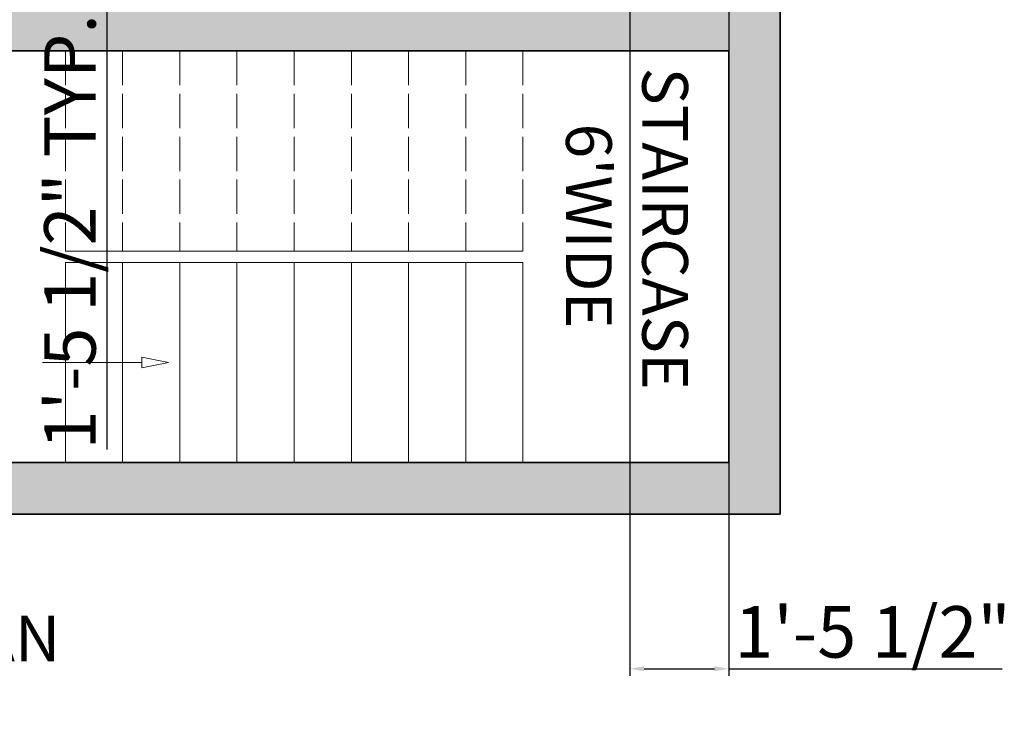
# Model space of a CAD drawing. Units: inches. Extents: x 3592 to 4861, y 1650 to 2243.
# Tile 11 of 30: x 4265 to 4438, y 1650 to 1772. Entities that reach past the tile are written whole.
import ezdxf

# ---------------------------------------------------------------- set-up
doc = ezdxf.new("R2010")
doc.units = ezdxf.units.IN
doc.linetypes.add('ACAD_ISO02W100', pattern=[15, 12, -3])
for name, color, linetype, lineweight in [('A-ANNO-DIMS', 2, 'Continuous', 13), ('A-ANNO-SYMB', 7, 'Continuous', 18), ('A-ANNO-TEXT', 7, 'Continuous', 25), ('A-AREA-IDEN', 7, 'Continuous', 18), ('A-FLOR-STRS', 7, 'Continuous', 18), ('A-FLOR-STRS-OVHD', 8, 'ACAD_ISO02W100', 13), ('A-WALL', 7, 'Continuous', 35)]:
    doc.layers.add(name, color=color, linetype=linetype, lineweight=lineweight)
doc.layers.add('A-WALL-PATT', color=252, linetype='Continuous', lineweight=13, true_color=0x939598)
doc.styles.get("Standard").update_dxf_attribs({"font": 'arial.ttf'})
doc.dimstyles.new('ISO-25', dxfattribs={"dimtxt": 9, "dimasz": 2.5, "dimexe": 1.25, "dimexo": 0.625, "dimtad": 1, "dimlunit": 3, "dimtxsty": 'Standard', "dimcen": 2.5, "dimadec": 0, "dimazin": 0, "dimtfac": 1, "dimtmove": 0, "dimatfit": 3, "dimfxl": 1, "dimarcsym": 0})

# ---------------------------------------------------------------- blocks, each defined once
blk = doc.blocks.new('ARROW-STAIR-DIRECTION')
blk.add_line((0, 0.94), (17.38, 0.94))
blk.add_lwpolyline([(22.04, 0.94), (17.38, 1.89), (17.38, 0)], close=True)
blk = doc.blocks.new('STAIR-LOWER-RUN')
for p, q in [((0, 35), (80, 35)), ((0, 35), (0, 0)), ((10, 35), (10, 0)), ((20, 35), (20, 0)), ((30, 35), (30, 0)), ((40, 35), (40, 0)), ((50, 35), (50, 0)), ((60, 35), (60, 0)), ((70, 35), (70, 0)), ((80, 35), (80, 0))]:
    blk.add_line(p, q)
blk = doc.blocks.new('STAIR-UPPER-RUN')
at = {"ltscale": 0.5}
for p, q in [((0, 35), (0, 0)), ((10, 35), (10, 0)), ((20, 35), (20, 0)), ((30, 35), (30, 0)), ((40, 35), (40, 0)), ((50, 35), (50, 0)), ((60, 35), (60, 0)), ((70, 35), (70, 0)), ((80, 35), (80, 0))]:
    blk.add_line(p, q, dxfattribs=at)
blk = doc.blocks.new('*D157')
at = {"layer": 'A-ANNO-DIMS', "color": 0, "lineweight": -2, "transparency": 16777216}
for p, q in [((4290.77, 1792.94), (4279.35, 1792.94)), ((4280.6, 1790.44), (4280.6, 1777.72)), ((4290.77, 1775.22), (4279.35, 1775.22)), ((4280.6, 1775.22), (4280.6, 1696.49))]:
    blk.add_line(p, q, dxfattribs=at)
at = {"layer": 'A-ANNO-DIMS', "color": 0, "transparency": 16777216}
for points in [[(4280.18, 1790.44), (4281.02, 1790.44), (4280.6, 1792.94)], [(4280.18, 1777.72), (4281.02, 1777.72), (4280.6, 1775.22)]]:
    blk.add_solid(points, dxfattribs=at)
at = {"layer": 'Defpoints', "color": 0, "transparency": 16777216}
for p in [(4291.39, 1792.94), (4280.6, 1775.22), (4291.39, 1775.22)]:
    blk.add_point(p, dxfattribs=at)
at = {"layer": 'A-ANNO-DIMS', "color": 0, "transparency": 16777216, "insert": (4275.32, 1734.6), "char_height": 9, "attachment_point": 5, "rotation": 90}
blk.add_mtext('1\'-5 1/2" TYP.', dxfattribs=at)
blk = doc.blocks.new('*D173')
at = {"layer": 'A-ANNO-DIMS', "color": 0, "lineweight": -2, "transparency": 16777216}
for p, q in [((4372.05, 2138.77), (4372.05, 1656.92)), ((4389.37, 2131.59), (4389.37, 1656.92)), ((4374.55, 1658.17), (4386.87, 1658.17)), ((4389.37, 1658.17), (4437.17, 1658.17))]:
    blk.add_line(p, q, dxfattribs=at)
at = {"layer": 'A-ANNO-DIMS', "color": 0, "transparency": 16777216}
for points in [[(4374.55, 1658.59), (4374.55, 1657.75), (4372.05, 1658.17)], [(4386.87, 1658.59), (4386.87, 1657.75), (4389.37, 1658.17)]]:
    blk.add_solid(points, dxfattribs=at)
at = {"layer": 'Defpoints', "color": 0, "transparency": 16777216}
for p in [(4372.05, 2139.4), (4389.37, 2132.22), (4389.37, 1658.17)]:
    blk.add_point(p, dxfattribs=at)
at = {"layer": 'A-ANNO-DIMS', "color": 0, "transparency": 16777216, "insert": (4414.52, 1663.45), "char_height": 9, "attachment_point": 5}
blk.add_mtext('1\'-5 1/2"', dxfattribs=at)

msp = doc.modelspace()

# ---------------------------------------------------------------- hatches: boundary and pattern name
at = {"layer": 'A-WALL-PATT'}
h = msp.add_hatch(color=256, dxfattribs=at)
h.dxf.hatch_style = 1
h.paths.add_polyline_path([(4398.37, 2165.219), (4038.37, 2165.219), (4038.37, 1993.219), (4047.37, 1993.219), (4047.37, 2156.219), (4191.37, 2156.219), (4191.37, 2150.219), (4195.37, 2150.219), (4195.37, 2156.219), (4256.37, 2156.219), (4256.37, 2150.219), (4265.37, 2150.219), (4265.37, 2156.219), (4389.37, 2156.219), (4389.37, 2114.219), (4398.37, 2114.219)])
h.paths.add_polyline_path([(4265.37, 2102.219), (4256.37, 2102.219), (4256.37, 2096.219), (4195.37, 2096.219), (4195.37, 2102.219), (4191.37, 2102.219), (4191.37, 2020.219), (4195.37, 2020.219), (4195.37, 2087.219), (4256.37, 2087.219), (4256.37, 2020.219), (4306.37, 2020.219), (4306.37, 2024.219), (4265.37, 2024.219)], flags=17)
h.paths.add_polyline_path([(4398.37, 2066.219), (4389.37, 2066.219), (4389.37, 2024.219), (4348.37, 2024.219), (4348.37, 2020.219), (4389.37, 2020.219), (4389.37, 1989.719), (4398.37, 1989.719)])
h.paths.add_polyline_path([(4398.37, 1941.719), (4389.37, 1941.719), (4389.37, 1911.219), (4301.37, 1911.219), (4301.37, 1907.219), (4389.37, 1907.219), (4389.37, 1865.219), (4398.37, 1865.219)])
h.paths.add_polyline_path([(4398.37, 1817.219), (4389.37, 1817.219), (4389.37, 1775.219), (4265.37, 1775.219), (4265.37, 1911.219), (4256.37, 1911.219), (4256.37, 1817.219), (4220.87, 1817.219), (4220.87, 1808.219), (4256.37, 1808.219), (4256.37, 1766.219), (4389.37, 1766.219), (4389.37, 1694.219), (4256.37, 1694.219), (4256.37, 1685.219), (4398.37, 1685.219)])
h.paths.add_polyline_path([(4178.87, 1817.219), (4077.37, 1817.219), (4077.37, 1808.219), (4178.87, 1808.219)])
h.paths.add_polyline_path([(4111.37, 2020.219), (4155.37, 2020.219), (4155.37, 2024.219), (4077.37, 2024.219), (4077.37, 2020.219), (4107.37, 2020.219), (4107.37, 1942.219), (4047.37, 1942.219), (4047.37, 1969.219), (4038.37, 1969.219), (4038.37, 1911.219), (4047.37, 1911.219), (4047.37, 1938.219), (4107.37, 1938.219), (4107.37, 1860.219), (4077.37, 1860.219), (4077.37, 1856.219), (4111.37, 1856.219)])
h.paths.add_polyline_path([(4047.37, 1887.219), (4038.37, 1887.219), (4038.37, 1685.219), (4152.37, 1685.219), (4152.37, 1715.219), (4143.37, 1715.219), (4143.37, 1694.219), (4047.37, 1694.219)])
h.paths.add_polyline_path([(4152.37, 1772.219), (4143.37, 1772.219), (4143.37, 1751.219), (4152.37, 1751.219)], flags=17)

# ---------------------------------------------------------------- linework, layer by layer
at = {"layer": 'A-FLOR-STRS'}
msp.add_line((4273.37, 1731.219), (4353.37, 1731.219), dxfattribs=at)
at = {"layer": 'A-WALL'}
for p, q in [((4398.37, 2165.219), (4398.37, 1685.219)), ((4389.37, 1766.219), (4256.37, 1766.219)), ((4389.37, 1766.219), (4389.37, 1694.219)), ((4389.37, 1694.219), (4256.37, 1694.219)), ((4398.37, 1685.219), (4256.37, 1685.219))]:
    msp.add_line(p, q, dxfattribs=at)

# ---------------------------------------------------------------- block references
at = {"layer": 'A-ANNO-SYMB'}
msp.add_blockref('ARROW-STAIR-DIRECTION', (4269.377, 1710.776), dxfattribs=at)
at = {"layer": 'A-FLOR-STRS'}
msp.add_blockref('STAIR-LOWER-RUN', (4273.369, 1694.219), dxfattribs=at)
at = {"layer": 'A-FLOR-STRS-OVHD'}
msp.add_blockref('STAIR-UPPER-RUN', (4273.369, 1731.219), dxfattribs=at)

# ---------------------------------------------------------------- texts
at = {"layer": 'A-ANNO-TEXT', "insert": (4159.302, 1667.444), "char_height": 8, "attachment_point": 1}
msp.add_mtext_dynamic_manual_height_columns('GROUND FLOOR PLAN', width=131.60551, gutter_width=12.5, heights=[0], dxfattribs=at)
at = {"layer": 'A-AREA-IDEN', "insert": (4382.242, 1763.303), "char_height": 8, "attachment_point": 1, "rotation": 270}
msp.add_mtext_dynamic_manual_height_columns("STAIRCASE\\P    6'WIDE", width=121.44943, gutter_width=12.5, heights=[0], dxfattribs=at)

# ---------------------------------------------------------------- dimensions: what is measured, and where the dimension line sits
at = {"layer": 'A-ANNO-DIMS'}
dim = msp.add_linear_dim(base=(4389.37, 1658.169), p1=(4372.046, 2139.399), p2=(4389.37, 2132.219), dimstyle='ISO-25', override={"dimdec": 1, "dimlfac": 1, "dimrnd": 0, "dimzin": 1, "dimdsep": 46, "dimlunit": 4, "dimfrac": 2}, dxfattribs=at)
dim.commit()
dim.dimension.update_dxf_attribs({"geometry": '*D173', "text_midpoint": (4414.519, 1663.447)})
dim = msp.add_linear_dim(base=(4280.6, 1775.219), p1=(4291.393, 1792.936), p2=(4291.393, 1775.219), angle=270, text='<> TYP.', dimstyle='ISO-25', override={"dimdec": 1, "dimlfac": 1, "dimrnd": 0, "dimzin": 1, "dimdsep": 46, "dimlunit": 4, "dimfrac": 2}, dxfattribs=at)
dim.commit()
dim.dimension.update_dxf_attribs({"geometry": '*D157', "text_midpoint": (4275.321, 1734.602)})

doc.saveas('drawing.dxf')
